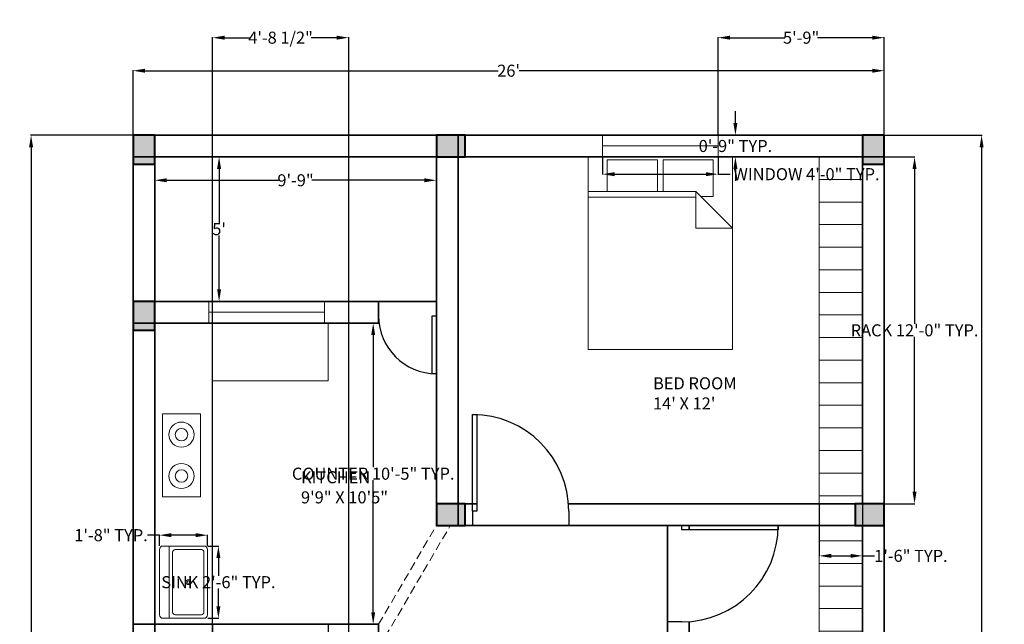
# Model space of a CAD drawing. Units: inches. Extents: x -54 to 881, y -122 to 681.
# Tile 6 of 6: x 472 to 881, y 421 to 672. Entities that reach past the tile are written whole.
import ezdxf

# ---------------------------------------------------------------- set-up
doc = ezdxf.new("R2010")
doc.units = ezdxf.units.IN
doc.header["$MEASUREMENT"] = 0
doc.linetypes.add('DASHED', pattern=[0.75, 0.5, -0.25])
for name, color, linetype, lineweight in [('A-ANNO-DIMS', 2, 'Continuous', 18), ('A-DOOR', 3, 'Continuous', 25), ('A-EQPM', 9, 'Continuous', 18), ('A-FLOR-CASE', 8, 'Continuous', 18), ('A-FLOR-FIXT', 9, 'Continuous', 18), ('A-FURN', 8, 'Continuous', 18), ('A-GLAZ', 4, 'Continuous', 20), ('A-WALL', 7, 'Continuous', 35), ('A-WALL-OVHD', 8, 'DASHED', 18)]:
    doc.layers.add(name, color=color, linetype=linetype, lineweight=lineweight)
doc.layers.add('A-AREA-IDEN', color=217, linetype='Continuous', lineweight=18, true_color=0x93278f)
doc.layers.add('A-COLS', color=240, linetype='Continuous', lineweight=40, true_color=0xed1f24)
doc.styles.get("Standard").update_dxf_attribs({"font": 'arial.ttf'})
doc.dimstyles.get("Standard").update_dxf_attribs({"dimtxt": 5, "dimasz": 5, "dimexe": 0.18, "dimexo": 0.0625, "dimgap": 0.09, "dimtad": 0, "dimtih": 1, "dimtoh": 1, "dimdec": 0, "dimzin": 0, "dimdsep": 46, "dimlunit": 3, "dimtxsty": 'Standard', "dimcen": 0.09, "dimadec": 0, "dimazin": 0, "dimtfac": 1, "dimtdec": 0, "dimtofl": 0, "dimtmove": 0, "dimatfit": 3, "dimfxl": 1, "dimtolj": 1, "dimtzin": 0, "dimarcsym": 0})

# ---------------------------------------------------------------- blocks, each defined once
blk = doc.blocks.new('*D15')
at = {"layer": 'A-ANNO-DIMS', "color": 0, "lineweight": -2, "transparency": 16777216}
for p, q in [((528.49, 614.94), (528.49, 605.09)), ((645.49, 614.94), (645.49, 605.09)), ((533.49, 605.27), (580.26, 605.27)), ((640.49, 605.27), (593.73, 605.27))]:
    blk.add_line(p, q, dxfattribs=at)
at = {"layer": 'A-ANNO-DIMS', "color": 0, "transparency": 16777216}
for points in [[(533.49, 606.11), (533.49, 604.44), (528.49, 605.27)], [(640.49, 606.11), (640.49, 604.44), (645.49, 605.27)]]:
    blk.add_solid(points, dxfattribs=at)
at = {"layer": 'Defpoints', "color": 0, "transparency": 16777216}
for p in [(528.49, 615), (645.49, 615), (645.49, 605.27)]:
    blk.add_point(p, dxfattribs=at)
at = {"layer": 'A-ANNO-DIMS', "color": 0, "transparency": 16777216, "insert": (586.99, 605.27), "char_height": 5, "attachment_point": 5}
blk.add_mtext('\\A1;9\'-9"', dxfattribs=at)
blk = doc.blocks.new('*D14')
at = {"layer": 'A-ANNO-DIMS', "color": 0, "lineweight": -2, "transparency": 16777216}
for p, q in [((519.43, 624), (476.98, 624)), ((477.16, 619), (477.16, 374.6)), ((477.16, 125), (477.16, 369.4)), ((519.43, 120), (476.98, 120))]:
    blk.add_line(p, q, dxfattribs=at)
at = {"layer": 'A-ANNO-DIMS', "color": 0, "transparency": 16777216}
for points in [[(476.32, 619), (477.99, 619), (477.16, 624)], [(476.32, 125), (477.99, 125), (477.16, 120)]]:
    blk.add_solid(points, dxfattribs=at)
at = {"layer": 'Defpoints', "color": 0, "transparency": 16777216}
for p in [(519.49, 624), (477.16, 120), (519.49, 120)]:
    blk.add_point(p, dxfattribs=at)
at = {"layer": 'A-ANNO-DIMS', "color": 0, "transparency": 16777216, "insert": (477.16, 372), "char_height": 5, "attachment_point": 5}
blk.add_mtext("\\A1;42'", dxfattribs=at)
blk = doc.blocks.new('*D16')
at = {"layer": 'A-ANNO-DIMS', "color": 0, "lineweight": -2, "transparency": 16777216}
for p, q in [((528.55, 615), (555.42, 615)), ((555.24, 610), (555.24, 587.63)), ((555.24, 560), (555.24, 582.37)), ((530.67, 555), (555.42, 555))]:
    blk.add_line(p, q, dxfattribs=at)
at = {"layer": 'A-ANNO-DIMS', "color": 0, "transparency": 16777216}
for points in [[(554.41, 610), (556.07, 610), (555.24, 615)], [(554.41, 560), (556.07, 560), (555.24, 555)]]:
    blk.add_solid(points, dxfattribs=at)
at = {"layer": 'Defpoints', "color": 0, "transparency": 16777216}
for p in [(528.49, 615), (530.61, 555), (555.24, 555)]:
    blk.add_point(p, dxfattribs=at)
at = {"layer": 'A-ANNO-DIMS', "color": 0, "transparency": 16777216, "insert": (555.24, 585), "char_height": 5, "attachment_point": 5}
blk.add_mtext("\\A1;5'", dxfattribs=at)
blk = doc.blocks.new('Sink-single - 30 in top')
blk.add_line((-15, -3.999996), (15, -3.999996))
for points in [[(-13.5, 0), (13.5, 0)], [(-15, -18.499996), (-15, -1.5)], [(15, -1.5), (15, -18.499996)], [(-13.5, -17.499996), (-13.5, -6.499996)], [(-12.5, -5.499996), (12.5, -5.499996)], [(13.5, -6.499996), (13.5, -17.499996)], [(13.5, -19.999996), (-13.5, -19.999996)], [(12.5, -18.499996), (-12.5, -18.499996)]]:
    blk.add_lwpolyline(points)
for radius in [1, 0.5]:
    blk.add_circle((0, -11.999996), radius)
for centre, radius, start, end in [((-13.5, -1.5), 1.5, 90, 180), ((13.5, -1.5), 1.5, 0, 90), ((-12.5, -6.499996), 1, 90, 180), ((12.5, -6.499996), 1, 0, 90), ((-13.5, -18.499996), 1.5, 180, 270), ((-12.5, -17.499996), 1, 180, 270), ((12.5, -17.499996), 1, 270, 0), ((13.5, -18.499996), 1.5, 270, 0)]:
    blk.add_arc(centre, radius, start, end)
blk = doc.blocks.new('Bed - Queen')
for p, q in [((0, -80.00003), (0, 0)), ((0, 0), (59.99999, 0)), ((59.99999, 0), (59.99999, -80.00003)), ((7.99999, -1.2), (28.79998, -1.2)), ((7.99999, -14.4), (7.99999, -1.2)), ((28.79998, -1.2), (28.79998, -14.4)), ((31.19999, -1.2), (51.99999, -1.2)), ((31.19999, -14.4), (31.19999, -1.2)), ((51.99999, -1.2), (51.99999, -16.4)), ((0, -14.4), (44.8, -14.4)), ((59.99999, -29.6), (44.8, -14.4)), ((44.8, -14.4), (44.8, -29.6)), ((44.8, -16.8), (0, -16.8)), ((51.99999, -16.4), (46.79936, -16.4)), ((44.8, -29.6), (59.99999, -29.6)), ((59.99999, -80.00003), (0, -80.00003))]:
    blk.add_line(p, q)
blk = doc.blocks.new('*U13')
for p, q in [((0, 0), (0, -6)), ((24, 0), (24, -6))]:
    blk.add_line(p, q)
blk.add_lwpolyline([(0, 0), (0, 24), (1.75, 24), (1.75, 0)], close=True)
blk.add_arc((0, 0), 24, 0, 90)
blk = doc.blocks.new('*U12')
for p, q in [((0, 0), (0, -6)), ((40, 0), (40, -6))]:
    blk.add_line(p, q)
blk.add_lwpolyline([(0, 0), (0, 40), (1.75, 40), (1.75, 0)], close=True)
blk.add_arc((0, 0), 40, 0, 90)
blk = doc.blocks.new('*D22')
at = {"layer": 'A-ANNO-DIMS', "color": 0, "lineweight": -2, "transparency": 16777216}
for p, q in [((519.49, 624.06), (519.49, 650.92)), ((524.49, 650.74), (671.12, 650.74)), ((826.49, 650.74), (679.87, 650.74)), ((831.49, 624.06), (831.49, 650.92))]:
    blk.add_line(p, q, dxfattribs=at)
at = {"layer": 'A-ANNO-DIMS', "color": 0, "transparency": 16777216}
for points in [[(524.49, 651.57), (524.49, 649.9), (519.49, 650.74)], [(826.49, 651.57), (826.49, 649.9), (831.49, 650.74)]]:
    blk.add_solid(points, dxfattribs=at)
at = {"layer": 'Defpoints', "color": 0, "transparency": 16777216}
for p in [(831.49, 650.74), (519.49, 624), (831.49, 624)]:
    blk.add_point(p, dxfattribs=at)
at = {"layer": 'A-ANNO-DIMS', "color": 0, "transparency": 16777216, "insert": (675.49, 650.74), "char_height": 5, "attachment_point": 5}
blk.add_mtext("\\A1;26'", dxfattribs=at)
blk = doc.blocks.new('WIN-48X9')
for p, q in [((0, 0), (0, 9)), ((48, 0), (48, 9)), ((0, 4.5), (48, 4.5))]:
    blk.add_line(p, q)
blk = doc.blocks.new('COOKTOP-2-BURNER')
blk.add_lwpolyline([(0, 34.35), (15.67, 34.35), (15.67, 0), (0, 0)], close=True)
for centre, radius in [((7.83, 25.76), 5.22), ((7.83, 25.76), 2.61), ((7.83, 8.59), 5.22), ((7.83, 8.59), 2.61)]:
    blk.add_circle(centre, radius)
blk = doc.blocks.new('KITCHEN-COUNTER-L')
for p, q in [((48, 101), (48, 125)), ((0, 0), (0, 101)), ((0, 101), (48, 101))]:
    blk.add_line(p, q)
blk = doc.blocks.new('STORAGE-RACK-144X18')
for p, q in [((0, 144), (18, 144)), ((0, 0), (0, 144)), ((0, 134.625), (18, 134.625)), ((0, 125.25), (18, 125.25)), ((0, 115.875), (18, 115.875)), ((0, 106.5), (18, 106.5)), ((0, 97.125), (18, 97.125)), ((0, 87.75), (18, 87.75)), ((0, 78.375), (18, 78.375)), ((0, 69), (18, 69)), ((0, 59.625), (18, 59.625)), ((0, 50.25), (18, 50.25)), ((0, 40.875), (18, 40.875)), ((0, 31.5), (18, 31.5)), ((0, 22.125), (18, 22.125)), ((0, 12.75), (18, 12.75)), ((0, 3.375), (18, 3.375))]:
    blk.add_line(p, q)
blk = doc.blocks.new('STORAGE-RACK-72X18')
for p, q in [((0, 0), (0, 72)), ((0, 65.625), (18, 65.625)), ((0, 56.25), (18, 56.25)), ((0, 46.875), (18, 46.875)), ((0, 37.5), (18, 37.5)), ((0, 28.125), (18, 28.125)), ((0, 18.75), (18, 18.75)), ((0, 9.375), (18, 9.375)), ((0, 0), (18, 0))]:
    blk.add_line(p, q)
blk = doc.blocks.new('COL-9X12')
h = blk.add_hatch(color=256)
h.dxf.hatch_style = 1
h.paths.add_polyline_path([(9, 12), (0, 12), (0, 0), (9, 0)])
blk.add_lwpolyline([(0, 0), (9, 0), (9, 12), (0, 12)], close=True)
blk = doc.blocks.new('*D42')
at = {"layer": 'A-ANNO-DIMS', "color": 0, "lineweight": -2, "transparency": 16777216}
for p, q in [((714.49, 614.94), (714.49, 607.62)), ((762.49, 614.94), (762.49, 607.62)), ((719.49, 607.8), (757.49, 607.8)), ((762.49, 607.8), (767.49, 607.8))]:
    blk.add_line(p, q, dxfattribs=at)
at = {"layer": 'A-ANNO-DIMS', "color": 0, "transparency": 16777216}
for points in [[(719.49, 608.63), (719.49, 606.97), (714.49, 607.8)], [(757.49, 608.63), (757.49, 606.97), (762.49, 607.8)]]:
    blk.add_solid(points, dxfattribs=at)
at = {"layer": 'Defpoints', "color": 0, "transparency": 16777216}
for p in [(714.49, 615), (762.49, 615), (762.49, 607.8)]:
    blk.add_point(p, dxfattribs=at)
at = {"layer": 'A-ANNO-DIMS', "color": 0, "transparency": 16777216, "insert": (799.22, 607.8), "char_height": 5, "attachment_point": 5}
blk.add_mtext('\\A1;WINDOW 4\'-0" TYP.', dxfattribs=at)
blk = doc.blocks.new('*D43')
at = {"layer": 'A-ANNO-DIMS', "color": 0, "lineweight": -2, "transparency": 16777216}
for p, q in [((769.69, 629), (769.69, 634)), ((762.55, 624), (769.87, 624)), ((762.55, 615), (769.87, 615)), ((769.69, 610), (769.69, 605))]:
    blk.add_line(p, q, dxfattribs=at)
at = {"layer": 'A-ANNO-DIMS', "color": 0, "transparency": 16777216}
for points in [[(768.86, 629), (770.52, 629), (769.69, 624)], [(768.86, 610), (770.52, 610), (769.69, 615)]]:
    blk.add_solid(points, dxfattribs=at)
at = {"layer": 'Defpoints', "color": 0, "transparency": 16777216}
for p in [(762.49, 624), (769.69, 624), (762.49, 615)]:
    blk.add_point(p, dxfattribs=at)
at = {"layer": 'A-ANNO-DIMS', "color": 0, "transparency": 16777216, "insert": (769.69, 619.5), "char_height": 5, "attachment_point": 5}
blk.add_mtext('\\A1;0\'-9" TYP.', dxfattribs=at)
blk = doc.blocks.new('*D56')
at = {"layer": 'A-ANNO-DIMS', "color": 0, "lineweight": -2, "transparency": 16777216}
for p, q in [((550.51, 453.48), (555.13, 453.48)), ((554.95, 448.48), (554.95, 441.16)), ((554.95, 428.48), (554.95, 435.81)), ((550.51, 423.48), (555.13, 423.48))]:
    blk.add_line(p, q, dxfattribs=at)
at = {"layer": 'A-ANNO-DIMS', "color": 0, "transparency": 16777216}
for points in [[(554.12, 448.48), (555.78, 448.48), (554.95, 453.48)], [(554.12, 428.48), (555.78, 428.48), (554.95, 423.48)]]:
    blk.add_solid(points, dxfattribs=at)
at = {"layer": 'Defpoints', "color": 0, "transparency": 16777216}
for p in [(550.45, 453.48), (554.95, 453.48), (550.45, 423.48)]:
    blk.add_point(p, dxfattribs=at)
at = {"layer": 'A-ANNO-DIMS', "color": 0, "transparency": 16777216, "insert": (554.95, 438.48), "char_height": 5, "attachment_point": 5}
blk.add_mtext('\\A1;SINK 2\'-6" TYP.', dxfattribs=at)
blk = doc.blocks.new('*D57')
at = {"layer": 'A-ANNO-DIMS', "color": 0, "lineweight": -2, "transparency": 16777216}
for p, q in [((530.45, 453.55), (530.45, 458.16)), ((550.45, 453.55), (550.45, 458.16)), ((530.45, 457.98), (525.45, 457.98)), ((545.45, 457.98), (535.45, 457.98))]:
    blk.add_line(p, q, dxfattribs=at)
at = {"layer": 'A-ANNO-DIMS', "color": 0, "transparency": 16777216}
for points in [[(535.45, 458.82), (535.45, 457.15), (530.45, 457.98)], [(545.45, 458.82), (545.45, 457.15), (550.45, 457.98)]]:
    blk.add_solid(points, dxfattribs=at)
at = {"layer": 'Defpoints', "color": 0, "transparency": 16777216}
for p in [(530.45, 457.98), (530.45, 453.48), (550.45, 453.48)]:
    blk.add_point(p, dxfattribs=at)
at = {"layer": 'A-ANNO-DIMS', "color": 0, "transparency": 16777216, "insert": (510.36, 457.98), "char_height": 5, "attachment_point": 5}
blk.add_mtext('\\A1;1\'-8" TYP.', dxfattribs=at)
blk = doc.blocks.new('*D66')
at = {"layer": 'A-ANNO-DIMS', "color": 0, "lineweight": -2, "transparency": 16777216}
for p, q in [((600.55, 546), (619.42, 546)), ((619.24, 541), (619.24, 486.18)), ((619.24, 426), (619.24, 480.82)), ((600.55, 421), (619.42, 421))]:
    blk.add_line(p, q, dxfattribs=at)
at = {"layer": 'A-ANNO-DIMS', "color": 0, "transparency": 16777216}
for points in [[(618.41, 541), (620.07, 541), (619.24, 546)], [(618.41, 426), (620.07, 426), (619.24, 421)]]:
    blk.add_solid(points, dxfattribs=at)
at = {"layer": 'Defpoints', "color": 0, "transparency": 16777216}
for p in [(600.49, 546), (619.24, 546), (600.49, 421)]:
    blk.add_point(p, dxfattribs=at)
at = {"layer": 'A-ANNO-DIMS', "color": 0, "transparency": 16777216, "insert": (619.24, 483.5), "char_height": 5, "attachment_point": 5}
blk.add_mtext('\\A1;COUNTER 10\'-5" TYP.', dxfattribs=at)
blk = doc.blocks.new('*D67')
at = {"layer": 'A-ANNO-DIMS', "color": 0, "lineweight": -2, "transparency": 16777216}
for p, q in [((552.49, 420.94), (552.49, 402.07)), ((600.49, 420.94), (600.49, 402.07)), ((557.49, 402.25), (561.06, 402.25)), ((595.49, 402.25), (591.92, 402.25))]:
    blk.add_line(p, q, dxfattribs=at)
at = {"layer": 'A-ANNO-DIMS', "color": 0, "transparency": 16777216}
for points in [[(557.49, 403.08), (557.49, 401.42), (552.49, 402.25)], [(595.49, 403.08), (595.49, 401.42), (600.49, 402.25)]]:
    blk.add_solid(points, dxfattribs=at)
at = {"layer": 'Defpoints', "color": 0, "transparency": 16777216}
for p in [(552.49, 421), (600.49, 421), (600.49, 402.25)]:
    blk.add_point(p, dxfattribs=at)
at = {"layer": 'A-ANNO-DIMS', "color": 0, "transparency": 16777216, "insert": (576.49, 402.25), "char_height": 5, "attachment_point": 5}
blk.add_mtext('\\A1;4\'-0" TYP.', dxfattribs=at)
blk = doc.blocks.new('*D68')
at = {"layer": 'A-ANNO-DIMS', "color": 0, "lineweight": -2, "transparency": 16777216}
for p, q in [((822.55, 615), (844.27, 615)), ((844.09, 610), (844.09, 545.68)), ((844.09, 476), (844.09, 540.32)), ((822.55, 471), (844.27, 471))]:
    blk.add_line(p, q, dxfattribs=at)
at = {"layer": 'A-ANNO-DIMS', "color": 0, "transparency": 16777216}
for points in [[(843.26, 610), (844.92, 610), (844.09, 615)], [(843.26, 476), (844.92, 476), (844.09, 471)]]:
    blk.add_solid(points, dxfattribs=at)
at = {"layer": 'Defpoints', "color": 0, "transparency": 16777216}
for p in [(822.49, 615), (844.09, 615), (822.49, 471)]:
    blk.add_point(p, dxfattribs=at)
at = {"layer": 'A-ANNO-DIMS', "color": 0, "transparency": 16777216, "insert": (844.09, 543), "char_height": 5, "attachment_point": 5}
blk.add_mtext('\\A1;RACK 12\'-0" TYP.', dxfattribs=at)
blk = doc.blocks.new('*D69')
at = {"layer": 'A-ANNO-DIMS', "color": 0, "lineweight": -2, "transparency": 16777216}
for p, q in [((804.49, 470.94), (804.49, 449.22)), ((822.49, 470.94), (822.49, 449.22)), ((809.49, 449.4), (817.49, 449.4)), ((822.49, 449.4), (827.49, 449.4))]:
    blk.add_line(p, q, dxfattribs=at)
at = {"layer": 'A-ANNO-DIMS', "color": 0, "transparency": 16777216}
for points in [[(809.49, 450.23), (809.49, 448.57), (804.49, 449.4)], [(817.49, 450.23), (817.49, 448.57), (822.49, 449.4)]]:
    blk.add_solid(points, dxfattribs=at)
at = {"layer": 'Defpoints', "color": 0, "transparency": 16777216}
for p in [(804.49, 471), (822.49, 471), (822.49, 449.4)]:
    blk.add_point(p, dxfattribs=at)
at = {"layer": 'A-ANNO-DIMS', "color": 0, "transparency": 16777216, "insert": (842.58, 449.4), "char_height": 5, "attachment_point": 5}
blk.add_mtext('\\A1;1\'-6" TYP.', dxfattribs=at)
blk = doc.blocks.new('*D75')
at = {"layer": 'A-ANNO-DIMS', "color": 0, "lineweight": -2, "transparency": 16777216}
for p, q in [((831.55, 624), (872.12, 624)), ((871.94, 619), (871.94, 350.64)), ((871.94, 77), (871.94, 345.36)), ((831.55, 72), (872.12, 72))]:
    blk.add_line(p, q, dxfattribs=at)
at = {"layer": 'A-ANNO-DIMS', "color": 0, "transparency": 16777216}
for points in [[(871.11, 619), (872.77, 619), (871.94, 624)], [(871.11, 77), (872.77, 77), (871.94, 72)]]:
    blk.add_solid(points, dxfattribs=at)
at = {"layer": 'Defpoints', "color": 0, "transparency": 16777216}
for p in [(831.49, 624), (871.94, 624), (831.49, 72)]:
    blk.add_point(p, dxfattribs=at)
at = {"layer": 'A-ANNO-DIMS', "color": 0, "transparency": 16777216, "insert": (871.94, 348), "char_height": 5, "attachment_point": 5}
blk.add_mtext('\\A1;46\'-0"', dxfattribs=at)
blk = doc.blocks.new('*D79')
at = {"layer": 'A-ANNO-DIMS', "color": 0, "lineweight": -2, "transparency": 16777216}
for p, q in [((552.49, 270.06), (552.49, 664.63)), ((557.49, 664.45), (568.12, 664.45)), ((604.07, 664.45), (593.44, 664.45)), ((609.07, 270.06), (609.07, 664.63))]:
    blk.add_line(p, q, dxfattribs=at)
at = {"layer": 'A-ANNO-DIMS', "color": 0, "transparency": 16777216}
for points in [[(557.49, 665.28), (557.49, 663.62), (552.49, 664.45)], [(604.07, 665.28), (604.07, 663.62), (609.07, 664.45)]]:
    blk.add_solid(points, dxfattribs=at)
at = {"layer": 'Defpoints', "color": 0, "transparency": 16777216}
for p in [(609.07, 664.45), (552.49, 270), (609.07, 270)]:
    blk.add_point(p, dxfattribs=at)
at = {"layer": 'A-ANNO-DIMS', "color": 0, "transparency": 16777216, "insert": (580.78, 664.45), "char_height": 5, "attachment_point": 5}
blk.add_mtext('\\A1;4\'-8 1/2"', dxfattribs=at)
blk = doc.blocks.new('*D81')
at = {"layer": 'A-ANNO-DIMS', "color": 0, "lineweight": -2, "transparency": 16777216}
for p, q in [((762.49, 624.06), (762.49, 664.63)), ((767.49, 664.45), (790.26, 664.45)), ((826.49, 664.45), (803.73, 664.45)), ((831.49, 624.06), (831.49, 664.63))]:
    blk.add_line(p, q, dxfattribs=at)
at = {"layer": 'A-ANNO-DIMS', "color": 0, "transparency": 16777216}
for points in [[(767.49, 665.28), (767.49, 663.62), (762.49, 664.45)], [(826.49, 665.28), (826.49, 663.62), (831.49, 664.45)]]:
    blk.add_solid(points, dxfattribs=at)
at = {"layer": 'Defpoints', "color": 0, "transparency": 16777216}
for p in [(831.49, 664.45), (762.49, 624), (831.49, 624)]:
    blk.add_point(p, dxfattribs=at)
at = {"layer": 'A-ANNO-DIMS', "color": 0, "transparency": 16777216, "insert": (796.99, 664.45), "char_height": 5, "attachment_point": 5}
blk.add_mtext('\\A1;5\'-9"', dxfattribs=at)

msp = doc.modelspace()

# ---------------------------------------------------------------- linework, layer by layer
at = {"layer": 'A-EQPM'}
msp.add_lwpolyline([(531.78, 508.3), (547.45, 508.3), (547.45, 473.95), (531.78, 473.95)], close=True, dxfattribs=at)
at = {"layer": 'A-FURN'}
msp.add_line((552.49, 305.1), (552.49, 421), dxfattribs=at)
at = {"layer": 'A-WALL'}
for p, q in [((519.49, 72), (519.49, 624)), ((519.49, 624), (831.49, 624)), ((528.49, 546), (528.49, 624)), ((645.49, 462), (645.49, 624)), ((654.49, 462), (654.49, 624)), ((831.49, 120), (831.49, 624)), ((519.49, 615), (654.49, 615)), ((654.49, 615), (831.49, 615)), ((822.49, 471), (822.49, 615)), ((519.49, 555), (645.49, 555)), ((621.49, 546), (621.49, 555)), ((519.49, 546), (621.49, 546)), ((528.49, 421), (528.49, 546)), ((654.49, 471), (662.24, 471)), ((700.38, 471), (831.49, 471)), ((654.49, 462), (645.49, 462)), ((654.49, 462), (831.49, 462)), ((741.49, 261), (741.49, 462)), ((750.49, 460.25), (750.49, 462)), ((822.49, 390), (822.49, 462)), ((750.49, 309.89), (750.49, 422.11)), ((519.49, 421), (621.49, 421)), ((528.49, 270), (528.49, 421)), ((621.49, 421), (621.49, 417))]:
    msp.add_line(p, q, dxfattribs=at)
at = {"layer": 'A-WALL-OVHD', "ltscale": 7}
for p, q in [((621.49, 421), (645.49, 462)), ((621.49, 411.1), (651.28, 462))]:
    msp.add_line(p, q, dxfattribs=at)

# ---------------------------------------------------------------- block references
at = {"layer": 'A-COLS'}
for p in [(519.49, 612), (822.49, 612), (519.49, 543)]:
    msp.add_blockref('COL-9X12', p, dxfattribs=at)
for p, rotation in [((645.49, 624), 269.9999999999995), ((645.49, 471), 269.9999999999995), ((819.49, 471), 269.9999999999984)]:
    msp.add_blockref('COL-9X12', p, dxfattribs=dict(at, rotation=rotation))
at = {"layer": 'A-DOOR'}
for name, p, rotation in [('*U13', (645.49, 549), 180), ('*U12', (747.49, 462), 270)]:
    msp.add_blockref(name, p, dxfattribs=dict(at, rotation=rotation))
msp.add_blockref('*U12', (660.49, 468), dxfattribs=at)
at = {"layer": 'A-EQPM'}
msp.add_blockref('COOKTOP-2-BURNER', (531.78, 473.95), dxfattribs=at)
at = {"layer": 'A-FLOR-CASE'}
for name, p in [('STORAGE-RACK-144X18', (804.49, 471)), ('KITCHEN-COUNTER-L', (552.49, 421)), ('STORAGE-RACK-72X18', (804.49, 390))]:
    msp.add_blockref(name, p, dxfattribs=at)
at = {"layer": 'A-FLOR-FIXT', "rotation": 90}
msp.add_blockref('Sink-single - 30 in top', (530.45, 438.48), dxfattribs=at)
at = {"layer": 'A-FURN'}
msp.add_blockref('Bed - Queen', (708.49, 615), dxfattribs=at)
at = {"layer": 'A-GLAZ'}
for p in [(714.49, 615), (550.99, 546.01)]:
    msp.add_blockref('WIN-48X9', p, dxfattribs=at)

# ---------------------------------------------------------------- texts
at = {"layer": 'A-AREA-IDEN', "char_height": 5, "attachment_point": 1}
for s, insert in [("BED ROOM\\P14' X 12'", (735.47, 523.5)), ('KITCHEN\\P9\'9" X 10\'5"', (589.26, 484.52))]:
    msp.add_mtext_dynamic_manual_height_columns(s, width=65.2326, gutter_width=1, heights=[0], dxfattribs=dict(at, insert=insert))

# ---------------------------------------------------------------- dimensions: what is measured, and where the dimension line sits
at = {"layer": 'A-ANNO-DIMS'}
for base, p1, p2, override, picture, middle in [((609.07, 664.45), (552.49, 270), (609.07, 270), {"dimdec": 1, "dimlfac": 1, "dimrnd": 0, "dimzin": 1, "dimdsep": 46, "dimlunit": 4, "dimfrac": 2}, '*D79', (580.78, 664.45)), ((831.49, 664.45), (762.49, 624), (831.49, 624), {"dimdec": 1, "dimlfac": 1, "dimrnd": 0, "dimzin": 1, "dimdsep": 46, "dimlunit": 4, "dimfrac": 2}, '*D81', (796.99, 664.45)), ((831.49, 650.74), (519.49, 624), (831.49, 624), {"dimclrd": 0, "dimclre": 0, "dimclrt": 0}, '*D22', (675.49, 650.74)), ((645.49, 605.27), (528.49, 615), (645.49, 615), {"dimclrd": 0, "dimclre": 0, "dimclrt": 0}, '*D15', (586.99, 605.27))]:
    dim = msp.add_linear_dim(base=base, p1=p1, p2=p2, dimstyle='Standard', override=override, dxfattribs=at)
    dim.commit()
    dim.dimension.update_dxf_attribs({"geometry": picture, "text_midpoint": middle})
for base, p1, p2, angle, text, picture, middle in [((769.69, 624), (762.49, 615), (762.49, 624), 90, '<> TYP.', '*D43', (769.69, 619.5)), ((844.09, 615), (822.49, 471), (822.49, 615), 90, 'RACK <> TYP.', '*D68', (844.09, 543)), ((619.24, 546), (600.49, 421), (600.49, 546), 90, 'COUNTER <> TYP.', '*D66', (619.24, 483.5)), ((530.45, 457.98), (550.45, 453.48), (530.45, 453.48), 180, '<> TYP.', '*D57', (510.36, 457.98)), ((554.95, 453.48), (550.45, 423.48), (550.45, 453.48), 90, 'SINK <> TYP.', '*D56', (554.95, 438.48))]:
    dim = msp.add_linear_dim(base=base, p1=p1, p2=p2, angle=angle, text=text, dimstyle='Standard', override={"dimdec": 1, "dimlfac": 1, "dimrnd": 0, "dimzin": 1, "dimdsep": 46, "dimlunit": 4, "dimfrac": 2}, dxfattribs=at)
    dim.commit()
    dim.dimension.update_dxf_attribs({"geometry": picture, "text_midpoint": middle})
for base, p1, p2, override, picture, middle in [((477.16, 120), (519.49, 624), (519.49, 120), {"dimclrd": 0, "dimclre": 0, "dimclrt": 0}, '*D14', (477.16, 372)), ((871.94, 624), (831.49, 72), (831.49, 624), {"dimdec": 1, "dimlfac": 1, "dimrnd": 0, "dimzin": 1, "dimdsep": 46, "dimlunit": 4, "dimfrac": 2}, '*D75', (871.94, 348)), ((555.24, 555), (528.49, 615), (530.61, 555), {"dimclrd": 0, "dimclre": 0, "dimclrt": 0}, '*D16', (555.24, 585))]:
    dim = msp.add_linear_dim(base=base, p1=p1, p2=p2, angle=90, dimstyle='Standard', override=override, dxfattribs=at)
    dim.commit()
    dim.dimension.update_dxf_attribs({"geometry": picture, "text_midpoint": middle})
for base, p1, p2, text, picture, middle in [((762.49, 607.8), (714.49, 615), (762.49, 615), 'WINDOW <> TYP.', '*D42', (799.22, 607.8)), ((822.49, 449.4), (804.49, 471), (822.49, 471), '<> TYP.', '*D69', (842.58, 449.4)), ((600.49, 402.25), (552.49, 421), (600.49, 421), '<> TYP.', '*D67', (576.49, 402.25))]:
    dim = msp.add_linear_dim(base=base, p1=p1, p2=p2, text=text, dimstyle='Standard', override={"dimdec": 1, "dimlfac": 1, "dimrnd": 0, "dimzin": 1, "dimdsep": 46, "dimlunit": 4, "dimfrac": 2}, dxfattribs=at)
    dim.commit()
    dim.dimension.update_dxf_attribs({"geometry": picture, "text_midpoint": middle})

doc.saveas('drawing.dxf')
